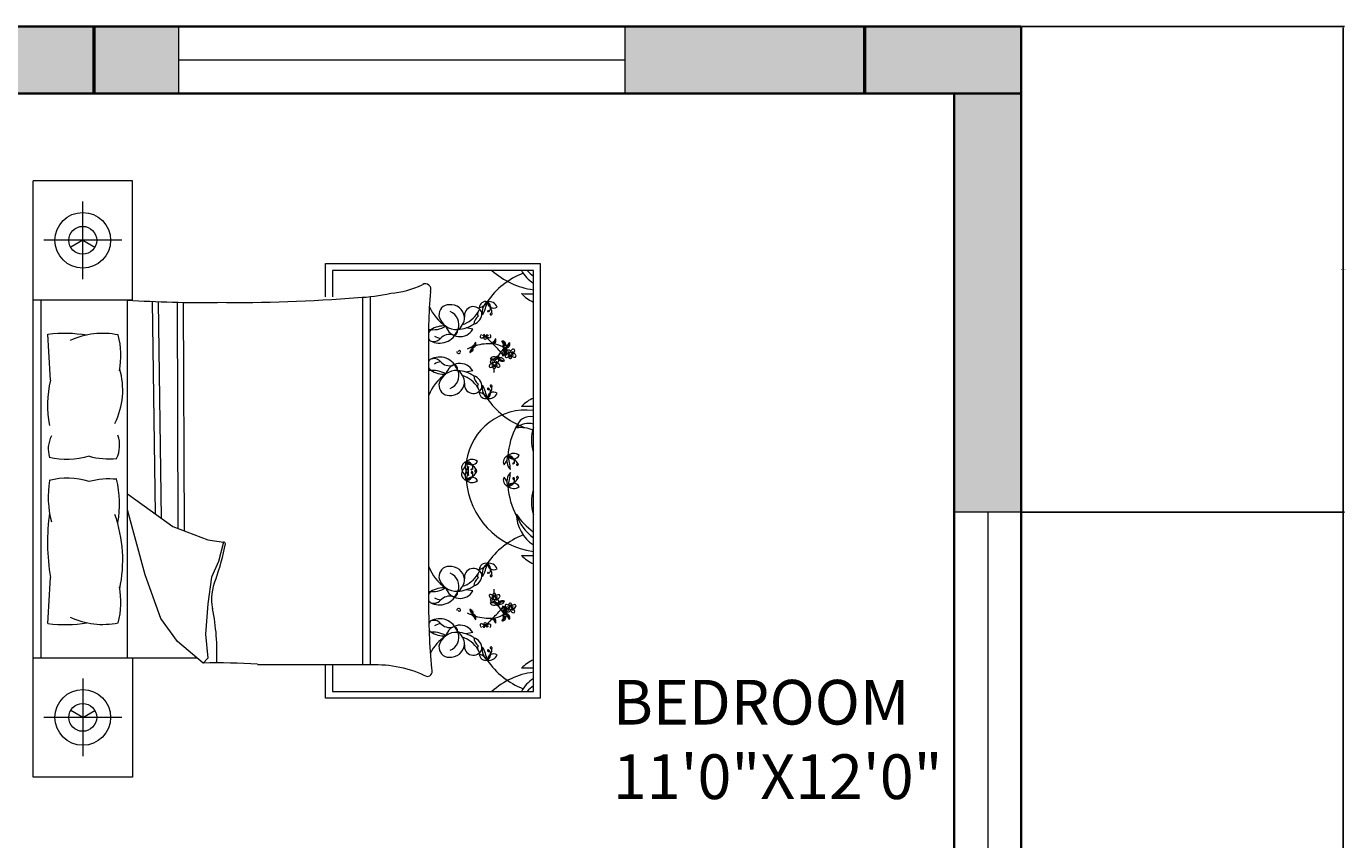
# Model space of a CAD drawing. Units: inches. Extents: x -28 to 485, y -861 to 54.
# Tile 14 of 14: x 308 to 485, y -99 to 10. Entities that reach past the tile are written whole.
import ezdxf

# ---------------------------------------------------------------- set-up
doc = ezdxf.new("R2010")
doc.units = ezdxf.units.IN
doc.header["$MEASUREMENT"] = 0
for name, color, linetype, lineweight in [('A-ANNO-DIMS', 2, 'Continuous', 18), ('A-AREA-IDEN', 7, 'Continuous', 18), ('A-COLS', 7, 'Continuous', 50), ('A-COLS-PATT', 8, 'Continuous', 13), ('A-FURN', 8, 'Continuous', 13), ('A-GLAZ', 4, 'Continuous', 18), ('A-WALL', 7, 'Continuous', 35), ('A-WALL-PATT', 34, 'Continuous', 13)]:
    doc.layers.add(name, color=color, linetype=linetype, lineweight=lineweight)
doc.styles.get("Standard").update_dxf_attribs({"font": 'arial.ttf'})
doc.dimstyles.get("Standard").update_dxf_attribs({"dimtxt": 0.18, "dimasz": 0.18, "dimexe": 0.18, "dimexo": 0.0625, "dimgap": 0.09, "dimtad": 0, "dimtih": 1, "dimtoh": 1, "dimdec": 0, "dimzin": 0, "dimdsep": 46, "dimlunit": 3, "dimtxsty": 'Standard', "dimcen": 0.09, "dimadec": 0, "dimazin": 0, "dimtfac": 1, "dimtdec": 0, "dimtofl": 0, "dimtmove": 0, "dimatfit": 3, "dimfxl": 1, "dimtolj": 1, "dimtzin": 0, "dimarcsym": 0})

# ---------------------------------------------------------------- blocks, each defined once
blk = doc.blocks.new('BED-DOUBLE-WITH-NIGHTSTANDS')
for p, q in [((0, 0), (0, 80.08)), ((6.67, 66.84), (6.67, 77.31)), ((11.91, 72.08), (1.44, 72.08)), ((39.26, 64.51), (39.26, 68.96)), ((39.26, 68.96), (68.11, 68.96)), ((40.19, 68.03), (40.19, 64.5)), ((67.18, 68.03), (40.19, 68.03)), ((67.18, 11.5), (67.18, 68.03)), ((68.11, 68.96), (68.11, 10.57)), ((1.03, 64.07), (1.03, 16.02)), ((12.66, 16.02), (12.66, 64.07)), ((15.98, 63.85), (16.38, 35.34)), ((16.8, 63.82), (17.22, 34.74)), ((19.33, 63.78), (19.45, 33.37)), ((20.15, 63.78), (20.27, 33.06)), ((44.25, 64.43), (44.25, 15.09)), ((45.25, 64.51), (45.25, 15.09)), ((59.06, 60.14), (58.15, 60.31)), ((53.12, 56.3), (53.12, 23.78)), ((59.06, 54.54), (58.15, 54.36)), ((12.66, 38.02), (18.76, 33.63)), ((15.04, 27.14), (12.66, 35.87)), ((18.76, 33.63), (23.47, 31.84)), ((23.47, 31.84), (25.57, 31.52)), ((25.57, 31.52), (24.92, 28.93)), ((24.92, 28.93), (23.95, 26.82)), ((17.14, 21.3), (15.04, 27.14)), ((23.95, 26.82), (23.47, 23.25)), ((59.06, 24.99), (58.15, 25.16)), ((23.47, 23.25), (23.14, 19.19)), ((19.41, 18.22), (17.14, 21.3)), ((22.82, 15.3), (19.41, 18.22)), ((23.14, 19.19), (23.47, 15.95)), ((59.06, 19.39), (58.15, 19.21)), ((0, 16.02), (21.98, 16.02)), ((23.47, 15.95), (22.82, 15.3)), ((39.26, 10.57), (39.26, 15.1)), ((40.19, 15.1), (40.19, 11.5)), ((6.67, 13.24), (6.67, 2.78)), ((40.19, 11.5), (67.18, 11.5)), ((68.11, 10.57), (39.26, 10.57)), ((11.91, 8.01), (1.44, 8.01))]:
    blk.add_line(p, q)
for points in [[(0, 64.07), (13.35, 64.07), (13.35, 80.08), (0, 80.08)], [(6.67, 72.08), (5.06, 71.14)], [(6.67, 72.08), (8.29, 71.14)], [(13.35, 16.02), (13.35, 0), (0, 0)], [(6.67, 8.01), (5.06, 8.94)], [(6.67, 8.01), (8.29, 8.94)]]:
    blk.add_lwpolyline(points)
for points in [[(43.62, 64.41, 0.056112), (48.03, 64.99, 0.095341), (52.27, 66.12)], [(2, 59.47, -0.074897), (7.23, 59.37, 0.472817)], [(7.52, 43.09, -0.14099), (2.18, 42.93, -0.235245)], [(7.52, 39.67, 0.14099), (2.18, 39.83, 0.235245)], [(2, 20.62, 0.074897), (7.23, 20.71, -0.472817)], [(30.15, 15.13, 0.001242), (45.35, 15.09, -0.127202), (52.92, 13.49)]]:
    blk.add_lwpolyline(points, format="xyb")
for centre, radius in [((6.67, 72.08), 3.74), ((6.67, 72.08), 1.87), ((64.11, 56.84), 0.204), ((61.96, 55.51), 0.204), ((61.96, 24.02), 0.204), ((64.11, 22.68), 0.204), ((6.67, 8.01), 3.74), ((6.67, 8.01), 1.87)]:
    blk.add_circle(centre, radius)
for centre, radius, start, end in [((69.62, 57.92), 10.46, 111.4092, 145.6135), ((68.59, 75.81), 10.46, 228.1144, 262.255), ((69.99, 70.57), 5.1, 209.8884, 236.5383), ((70.94, 72.4), 6.35, 223.5186, 233.6964), ((52.68, 65.51), 0.73, 336.5219, 123.8264), ((22.44, 207.63), 143.9, 266.1, 270.9282), ((27.68, 251.44), 187.71, 269.1145, 274.8735), ((131.01, 58.75), 77.93, 175.2402, 181.8035), ((60.79, 62.99), 0.867, 76.272, 177.0484), ((59.47, 64.76), 1.79, 284.7031, 328.6173), ((61.96, 62.49), 1.65, 125.7657, 194.5347), ((53.85, 65.41), 7.32, 332.8176, 347.4827), ((61.24, 62.69), 1.16, 20.9613, 102.2885), ((61.86, 63.85), 0.873, 181.7131, 301.5367), ((59, 62.09), 2.64, 2.0648, 41.1598), ((60.59, 63.07), 0.856, 316.2238, 62.3173), ((68.81, 67.71), 4.25, 221.0454, 247.4453), ((66.52, 79.36), 14.47, 266.3481, 272.5919), ((58.76, 65.61), 6.06, 203.6453, 236.3329), ((55.85, 62.08), 1.35, 88.9462, 185.5144), ((56.04, 61.53), 1.91, 7.1143, 95.0551), ((55.32, 60.77), 1.86, 338.5779, 68.4181), ((56.48, 64.35), 3.78, 288.2955, 328.7386), ((59.12, 61.97), 1.2, 19.1312, 189.736), ((58.76, 62.26), 1.5, 285.6955, 4.031), ((60.43, 62.21), 0.737, 126.7319, 206.0245), ((61.09, 62.57), 0.0682, 20.2667, 316.2271), ((61.51, 62.18), 0.13, 168.5166, 2.0648), ((61.45, 62.19), 0.0631, 52.0591, 168.5166), ((53.71, 63.39), 3.32, 259.249, 301.1782), ((55.15, 57.49), 3.09, 85.2696, 124.215), ((56.85, 62.5), 2.41, 193.079, 274.7067), ((57.33, 61.13), 1.99, 196.8663, 330.0915), ((55.62, 61.86), 2.33, 305.9599, 357.6409), ((56.78, 64.39), 4.3, 273.4924, 303.7117), ((60.76, 60.64), 1.6, 128.4175, 173.8338), ((-760.15, 15.33), 763.42, 2.85022, 3.31479), ((9.33, 49.26), 10.32, 78.2417, 114.8684), ((1.06, 56.61), 10.73, 348.9631, 14.8961), ((54, 59.28), 0.964, 127.675, 162.5814), ((54, 59.28), 0.964, 196.6343, 225.5483), ((54.57, 60.82), 2.55, 240.8249, 340.7178), ((53.81, 59.69), 1.2, 246.1646, 318.4347), ((55.03, 61.2), 2.3, 240.0851, 262.564), ((55.94, 57.8), 1.64, 74.8529, 138.4347), ((56.5, 59.87), 0.497, 254.8529, 12.6959), ((55.15, 57.49), 3.09, 53.6555, 57.2989), ((60.19, 59.12), 0.158, 125.0752, 284.7644), ((60.43, 59.18), 0.34, 127.3642, 168.4363), ((60.17, 59.45), 0.49, 277.4968, 341.2737), ((60.56, 59.22), 0.195, 88.1325, 178.8919), ((60.95, 59.02), 0.422, 136.3462, 189.6513), ((60.71, 58.98), 0.176, 189.6513, 312.3208), ((60.75, 59.46), 0.204, 183.2768, 356.7232), ((61.39, 59.1), 0.668, 164.2829, 186.9148), ((60.6, 59.09), 0.334, 312.3208, 40.2111), ((61.31, 59.47), 0.474, 201.6382, 274.947), ((60.68, 58.82), 0.619, 42.3896, 66.5724), ((66.93, 63.72), 7.6, 217.9541, 226.8459), ((61.13, 59.18), 0.337, 10.9597, 52.2379), ((61.33, 59.15), 0.156, 274.947, 37.5263), ((61.75, 58.56), 0.384, 265.7131, 351.6568), ((60.91, 59.35), 1.29, 313.6929, 321.7899), ((62.33, 58.47), 0.42, 115.5379, 168.6744), ((60.9, 59.07), 1.27, 329.344, 349.7412), ((59.89, 58.78), 2.26, 352.8698, 1.6736), ((63.07, 58.33), 0.228, 33.0979, 123.1364), ((58.05, 55.12), 5.96, 31.1156, 34.8118), ((62.74, 57.94), 0.617, 2.3172, 70.5201), ((57.16, 57.12), 0.251, 169.5864, 349.5616), ((57.25, 57.11), 0.154, 349.5616, 167.2949), ((61.28, 51.56), 6.63, 110.1059, 116.9968), ((59.06, 57.02), 0.42, 129.5056, 182.6421), ((57.85, 58), 1.27, 308.4388, 328.836), ((57.63, 59.02), 2.26, 296.5064, 305.3102), ((57.61, 57.86), 1.29, 336.3901, 344.4871), ((59.01, 57.53), 0.163, 83.9457, 185.6216), ((58.36, 57.69), 0.671, 328.836, 0.8141), ((58.71, 57.49), 0.384, 306.5232, 32.4668), ((59.16, 57.79), 0.163, 112.5583, 214.2343), ((59.06, 58.08), 0.384, 265.7131, 351.6568), ((58.72, 58.29), 0.671, 297.3659, 329.344), ((58.21, 58.87), 1.29, 313.6929, 321.7899), ((59.64, 57.99), 0.42, 115.5379, 168.6744), ((58.21, 58.6), 1.27, 329.344, 349.7412), ((61.28, 51.56), 6.63, 86.1723, 106.4158), ((57.2, 58.31), 2.26, 352.8698, 1.6736), ((61.86, 58.27), 0.163, 112.5583, 214.2343), ((61.42, 58.77), 0.671, 297.3659, 329.344), ((61.45, 54.86), 3.33, 60.7959, 85.244), ((54.37, 50.07), 10.94, 37.8256, 47.7588), ((65.87, 54.52), 3.99, 130.182, 149.456), ((63.67, 56.79), 0.658, 139.3812, 199.9959), ((62.44, 57.27), 0.93, 310.9365, 22.7695), ((62.87, 57.22), 0.675, 285.6484, 332.2957), ((63.25, 57.78), 0.178, 135.7354, 318.1297), ((62.95, 58.07), 0.236, 315.7354, 31.1156), ((62.75, 57.57), 0.547, 319.3812, 5.5456), ((63.38, 57.79), 0.178, 68.2452, 250.6395), ((62.97, 58), 0.531, 352.6008, 57.1845), ((64.87, 54.44), 3.55, 111.7087, 116.2181), ((61.45, 54.86), 3.33, 47.5083, 55.9967), ((63.48, 58.12), 0.531, 252.8042, 349.6943), ((62.97, 57.17), 0.565, 331.1838, 51.6792), ((63.53, 58.17), 0.236, 248.2452, 323.6254), ((63.8, 56.56), 0.34, 93.635, 168.4363), ((63.33, 58.31), 0.617, 291.7087, 3.0299), ((63.75, 57.1), 0.2, 138.2946, 276.2474), ((63.83, 57.07), 0.278, 358.5719, 143.8954), ((58.93, 61.56), 5.96, 323.6254, 327.3216), ((63.92, 56.61), 0.195, 88.1325, 178.8919), ((63.99, 57.29), 0.281, 208.8493, 269.9355), ((63.75, 57.22), 0.321, 274.2123, 318.1587), ((63.81, 58.16), 0.228, 325.6077, 55.6462), ((64.73, 56.9), 0.643, 121.9501, 165.2442), ((64.28, 57.14), 0.135, 262.868, 7.094), ((64.04, 56.2), 0.619, 42.3896, 66.5724), ((64.27, 57.26), 0.403, 278.5614, 22.5914), ((64.49, 56.56), 0.337, 10.9597, 118.7804), ((64.49, 57.27), 0.202, 44.3732, 121.9501), ((54, 55.39), 0.964, 134.4517, 156.7144), ((54, 55.39), 0.964, 203.2856, 232.325), ((54.57, 53.85), 2.55, 19.2822, 119.1751), ((53.81, 54.99), 1.2, 41.5653, 113.8354), ((55.03, 53.47), 2.3, 97.436, 119.9149), ((55.94, 56.87), 1.64, 221.5653, 285.1471), ((57.33, 53.55), 1.99, 29.9085, 163.1337), ((56.5, 54.81), 0.497, 347.3041, 105.1471), ((61.4, 55.17), 0.158, 125.0752, 284.7644), ((61.65, 55.23), 0.34, 93.635, 168.4363), ((61.66, 57.07), 0.93, 253.6301, 325.4631), ((61.92, 55.78), 0.658, 82.0748, 142.6895), ((61.85, 56.68), 0.675, 228.342, 274.9894), ((61.6, 55.76), 0.2, 138.2946, 276.2474), ((61.38, 55.5), 0.49, 277.4968, 341.2737), ((61.68, 55.73), 0.278, 358.5719, 143.8954), ((61.77, 55.27), 0.195, 88.1325, 178.8919), ((61.84, 55.95), 0.281, 208.8493, 269.9355), ((61.6, 55.89), 0.321, 274.2123, 318.1587), ((62.16, 55.06), 0.422, 136.3462, 189.6513), ((61.92, 55.02), 0.176, 189.6513, 312.3208), ((61.87, 56.57), 0.565, 273.8774, 357.1501), ((62.6, 55.14), 0.668, 164.2829, 186.9148), ((62.58, 55.56), 0.643, 121.9501, 165.2442), ((62.09, 56.97), 0.547, 262.0748, 308.2393), ((61.81, 55.14), 0.334, 312.3208, 40.2111), ((62.52, 55.52), 0.474, 201.6382, 274.947), ((62.13, 55.81), 0.135, 262.868, 7.094), ((61.89, 54.87), 0.619, 42.3896, 66.5724), ((62.12, 55.92), 0.403, 278.5614, 22.5914), ((62.34, 55.23), 0.337, 10.9597, 118.7804), ((65.87, 54.52), 3.99, 156.1523, 156.9499), ((62.34, 55.94), 0.202, 44.3732, 121.9501), ((62.97, 56.41), 0.565, 181.4625, 249.4747), ((62.87, 56.86), 0.547, 215.1128, 261.2773), ((63.31, 56.83), 0.93, 197.889, 269.722), ((62.55, 55.2), 0.156, 274.947, 37.5263), ((63.02, 56.51), 0.675, 248.3627, 295.0101), ((62.69, 55.67), 0.658, 20.6625, 81.2773), ((63.55, 56.5), 0.158, 125.0752, 284.7644), ((63.53, 56.83), 0.49, 277.4968, 341.2737), ((64.31, 56.4), 0.422, 136.3462, 189.6513), ((64.07, 56.36), 0.176, 189.6513, 312.3208), ((64.75, 56.48), 0.668, 164.2829, 186.9148), ((63.96, 56.47), 0.334, 312.3208, 40.2111), ((64.67, 56.85), 0.474, 201.6382, 274.947), ((64.7, 56.53), 0.156, 274.947, 37.5263), ((16.01, 49.96), 14.08, 166.3427, 191.1841), ((1.85, 51.98), 10.19, 333.8761, 16.1746), ((53.71, 51.28), 3.32, 58.8218, 100.2867), ((58.76, 49.06), 6.06, 123.6671, 158.5059), ((55.15, 57.18), 3.09, 235.785, 274.7304), ((56.85, 52.18), 2.41, 85.2933, 166.921), ((55.32, 53.9), 1.86, 291.5819, 21.4221), ((55.15, 57.18), 3.09, 302.7011, 306.3445), ((55.62, 52.81), 2.33, 2.3591, 54.0401), ((56.78, 50.29), 4.3, 56.2883, 86.5076), ((56.48, 50.32), 3.78, 31.2614, 71.7045), ((60.76, 54.03), 1.6, 186.1662, 231.5825), ((58.76, 52.42), 1.5, 355.969, 74.3045), ((65.87, 54.52), 3.99, 175.2415, 182.8929), ((55.85, 52.59), 1.35, 174.4856, 271.0538), ((56.04, 53.15), 1.91, 264.9449, 352.8857), ((59.12, 52.71), 1.2, 170.264, 340.8688), ((60.43, 52.46), 0.737, 153.9755, 233.2681), ((60.79, 51.69), 0.867, 182.9516, 283.728), ((59.47, 49.92), 1.79, 31.3827, 75.2969), ((61.96, 52.19), 1.65, 165.4653, 234.2343), ((53.85, 49.26), 7.32, 12.5173, 27.1824), ((59, 52.59), 2.64, 318.8402, 357.9352), ((60.59, 51.6), 0.856, 297.6827, 43.7762), ((61.86, 50.82), 0.873, 58.4633, 178.2869), ((61.24, 51.98), 1.16, 257.7115, 339.0387), ((61.13, 52.12), 0.113, 43.7762, 339.7183), ((61.51, 52.5), 0.13, 357.9352, 191.4834), ((61.45, 52.48), 0.0631, 191.4834, 307.9409), ((69.62, 56.75), 10.46, 214.3865, 248.5908), ((68.81, 46.96), 4.25, 112.5547, 138.9546), ((66.52, 35.31), 14.47, 87.4081, 93.6519), ((66.17, 41.19), 8.09, 82.8636, 171.8197), ((66.74, 46.53), 1.88, 76.3898, 169.0739), ((74.19, 42.33), 10.46, 152.5854, 175.5377), ((66.48, 45.12), 2.37, 72.8609, 131.9049), ((65.43, 42.24), 4.68, 68.117, 96.6195), ((72.68, 45.26), 5.75, 162.9798, 196.4569), ((5.99, 44.03), 3.96, 153.3437, 196.1026), ((7.37, 44.56), 4.25, 335.0183, 18.5407), ((10.2, 52.53), 9.81, 254.1707, 275.9871), ((58.94, 41.49), 1.16, 50.8855, 132.2127), ((64.01, 42.31), 0.867, 106.1963, 206.9726), ((61.98, 43.19), 1.79, 314.6273, 358.5415), ((65.27, 42.46), 1.65, 155.6899, 224.4589), ((64.54, 42.29), 1.16, 50.8855, 132.2127), ((64.51, 43.6), 0.873, 211.6373, 331.4609), ((63.8, 42.29), 0.856, 346.148, 92.2415), ((62.91, 40.64), 2.64, 31.989, 71.0841), ((56.78, 40.96), 7.32, 2.7418, 17.407), ((75.64, 42.98), 8.5, 174.3643, 175.6213), ((81.47, 38.5), 15.2, 160.0972, 160.2783), ((58.4, 41.51), 0.867, 106.1963, 206.9726), ((58.4, 40.68), 0.867, 153.0274, 253.8037), ((56.38, 42.39), 1.79, 314.6273, 358.5415), ((56.38, 39.81), 1.79, 1.4585, 45.3727), ((59.67, 41.66), 1.65, 155.6899, 224.4589), ((59.67, 40.53), 1.65, 135.5411, 204.3101), ((58.91, 42.8), 0.873, 211.6373, 331.4609), ((58.2, 41.49), 0.856, 346.148, 92.2415), ((57.3, 39.84), 2.64, 31.989, 71.0841), ((51.18, 40.16), 7.32, 2.7418, 17.407), ((51.18, 42.04), 7.32, 342.593, 357.2582), ((57.3, 42.35), 2.64, 288.9159, 328.011), ((58.2, 40.71), 0.856, 267.7585, 13.852), ((58.87, 41.3), 0.0682, 50.1909, 346.0209), ((58.92, 40.88), 0.113, 13.852, 309.9245), ((59.44, 41.17), 0.13, 198.4408, 31.989), ((59.37, 41.15), 0.0631, 81.9833, 198.4408), ((59.44, 41.02), 0.13, 328.011, 161.5592), ((59.37, 41.04), 0.0631, 161.5592, 278.0167), ((65.27, 39.73), 1.65, 135.5411, 204.3101), ((56.78, 41.24), 7.32, 342.593, 357.2582), ((64.47, 42.1), 0.0682, 50.1909, 346.0209), ((64.98, 41.95), 0.0631, 81.9833, 198.4408), ((65.04, 41.98), 0.13, 198.4408, 31.989), ((16.3, 37.72), 14.27, 171.5249, 193.96), ((10.2, 30.23), 9.81, 84.0129, 105.8293), ((-2.51, 36.66), 14.12, 349.8617, 13.6238), ((58.91, 39.39), 0.873, 28.5391, 148.3627), ((58.94, 40.71), 1.16, 227.7873, 309.1145), ((68.59, 40.66), 10.46, 184.4623, 262.255), ((64.01, 39.88), 0.867, 153.0274, 253.8037), ((61.98, 39.01), 1.79, 1.4585, 45.3727), ((62.91, 41.55), 2.64, 288.9159, 328.011), ((63.8, 39.91), 0.856, 267.7585, 13.852), ((64.51, 38.59), 0.873, 28.5391, 148.3627), ((64.54, 39.91), 1.16, 227.7873, 309.1145), ((74.19, 39.86), 10.46, 184.4623, 207.4146), ((64.52, 40.08), 0.113, 13.852, 309.9245), ((64.98, 40.24), 0.0631, 161.5592, 278.0167), ((65.04, 40.22), 0.13, 328.011, 161.5592), ((72.68, 36.94), 5.75, 163.5431, 197.0202), ((75.64, 39.22), 8.5, 184.3787, 185.6357), ((81.47, 43.7), 15.2, 199.7217, 199.9028), ((30.98, 31.59), 29.04, 172.2196, 189.497), ((-6.57, 29.12), 18.61, 348.0397, 19.2615), ((69.99, 35.42), 5.1, 181.272, 236.5383), ((72.72, 40.59), 9.45, 214.0123, 234.053), ((70.94, 37.25), 6.35, 197.8504, 233.6964), ((69.62, 22.77), 10.46, 111.4092, 145.6135), ((-4.69, 37.08), 31.06, 340.1194, 349.3383), ((25.64, 31.34), 0.193, 358.8623, 109.7536), ((60.79, 27.84), 0.867, 76.272, 177.0484), ((59.47, 29.61), 1.79, 284.7031, 328.6173), ((61.96, 27.34), 1.65, 125.7657, 194.5347), ((53.85, 30.27), 7.32, 332.8176, 347.4827), ((61.24, 27.55), 1.16, 20.9613, 102.2885), ((60.59, 27.92), 0.856, 316.2238, 62.3173), ((59, 26.94), 2.64, 2.0648, 41.1598), ((61.86, 28.71), 0.873, 181.7131, 301.5367), ((66.52, 44.21), 14.47, 266.3481, 272.5919), ((68.81, 32.56), 4.25, 221.0454, 247.4453), ((-760.15, 64.76), 763.42, 356.68521, 357.14978), ((58.76, 30.46), 6.06, 201.4941, 236.3329), ((55.85, 26.93), 1.35, 88.9462, 185.5144), ((56.85, 27.35), 2.41, 193.079, 274.7067), ((56.04, 26.38), 1.91, 7.1143, 95.0551), ((55.32, 25.63), 1.86, 338.5779, 68.4181), ((55.62, 26.71), 2.33, 305.9599, 357.6409), ((56.48, 29.2), 3.78, 288.2955, 328.7386), ((59.12, 26.82), 1.2, 19.1312, 189.736), ((58.76, 27.11), 1.5, 285.6955, 4.031), ((60.76, 25.49), 1.6, 128.4175, 173.8338), ((60.43, 27.07), 0.737, 126.7319, 206.0245), ((61.09, 27.42), 0.0682, 20.2667, 316.2271), ((61.51, 27.03), 0.13, 168.5166, 2.0648), ((61.45, 27.04), 0.0631, 52.0591, 168.5166), ((1.06, 23.47), 10.73, 345.1039, 11.0369), ((30.48, 23.89), 6.52, 156.2616, 191.3392), ((53.71, 28.24), 3.32, 259.7133, 301.1782), ((54, 24.13), 0.964, 127.675, 156.7144), ((54.57, 25.67), 2.55, 240.8249, 340.7178), ((55.15, 22.34), 3.09, 85.2696, 124.215), ((57.33, 25.98), 1.99, 196.8663, 330.0915), ((56.5, 24.72), 0.497, 254.8529, 12.6959), ((55.15, 22.34), 3.09, 53.6555, 57.2989), ((56.78, 29.24), 4.3, 273.4924, 303.7117), ((65.87, 25.01), 3.99, 177.1071, 184.7585), ((136.48, 22.83), 83.37, 179.3433, 185.6887), ((54, 24.13), 0.964, 203.229, 225.5483), ((53.81, 24.54), 1.2, 246.1646, 318.4347), ((55.03, 26.06), 2.3, 240.0851, 262.564), ((55.94, 22.65), 1.64, 74.8529, 138.4347), ((61.4, 24.36), 0.158, 75.2356, 234.9248), ((61.65, 24.3), 0.34, 191.5637, 266.365), ((61.6, 23.76), 0.2, 83.7526, 221.7054), ((61.85, 22.84), 0.675, 85.0106, 131.658), ((61.66, 22.46), 0.93, 34.5369, 106.3699), ((61.92, 23.75), 0.658, 217.3105, 277.9252), ((61.38, 24.03), 0.49, 18.7263, 82.5032), ((61.68, 23.79), 0.278, 216.1046, 1.4281), ((61.77, 24.25), 0.195, 181.1081, 271.8675), ((61.84, 23.57), 0.281, 90.0645, 151.1507), ((61.6, 23.64), 0.321, 41.8413, 85.7877), ((61.92, 24.5), 0.176, 47.6792, 170.3487), ((62.16, 24.46), 0.422, 170.3487, 223.6538), ((61.87, 22.95), 0.565, 2.8499, 86.1226), ((62.6, 24.38), 0.668, 173.0852, 195.7171), ((62.58, 23.96), 0.643, 194.7558, 238.0499), ((62.09, 22.55), 0.547, 51.7607, 97.9252), ((61.81, 24.39), 0.334, 319.7889, 47.6792), ((62.52, 24.01), 0.474, 85.053, 158.3618), ((62.13, 23.71), 0.135, 352.906, 97.132), ((61.89, 24.66), 0.619, 293.4276, 317.6104), ((62.34, 24.29), 0.337, 241.2196, 349.0403), ((62.12, 23.6), 0.403, 337.4086, 81.4386), ((65.87, 25.01), 3.99, 203.0501, 203.8477), ((62.34, 23.59), 0.202, 238.0499, 315.6268), ((62.97, 23.11), 0.565, 110.5253, 178.5375), ((63.31, 22.7), 0.93, 90.278, 162.111), ((62.87, 22.67), 0.547, 98.7227, 144.8872), ((62.55, 24.33), 0.156, 322.4737, 85.053), ((63.02, 23.01), 0.675, 64.9899, 111.6373), ((62.69, 23.86), 0.658, 278.7227, 339.3375), ((63.55, 23.03), 0.158, 75.2356, 234.9248), ((63.53, 22.69), 0.49, 18.7263, 82.5032), ((64.07, 23.17), 0.176, 47.6792, 170.3487), ((64.31, 23.13), 0.422, 170.3487, 223.6538), ((64.75, 23.05), 0.668, 173.0852, 195.7171), ((63.96, 23.05), 0.334, 319.7889, 47.6792), ((64.67, 22.68), 0.474, 85.053, 158.3618), ((64.7, 22.99), 0.156, 322.4737, 85.053), ((9.33, 30.82), 10.32, 245.1316, 281.7583), ((-5.54, 16.67), 30.23, 357.4519, 11.3392), ((57.16, 22.4), 0.251, 10.4384, 190.4136), ((57.25, 22.42), 0.154, 192.7051, 10.4384), ((61.28, 27.97), 6.63, 243.0032, 249.8941), ((57.85, 21.53), 1.27, 31.164, 51.5612), ((59.06, 22.5), 0.42, 177.3579, 230.4944), ((57.63, 20.5), 2.26, 54.6898, 63.4936), ((57.61, 21.66), 1.29, 15.5129, 23.6099), ((59.01, 21.99), 0.163, 174.3784, 276.0543), ((58.71, 22.03), 0.384, 327.5332, 53.4768), ((58.36, 21.84), 0.671, 359.1859, 31.164), ((59.16, 21.74), 0.163, 145.7657, 247.4417), ((59.06, 21.45), 0.384, 8.3432, 94.2869), ((58.72, 21.23), 0.671, 30.656, 62.6341), ((58.21, 20.66), 1.29, 38.2101, 46.3071), ((59.64, 21.53), 0.42, 191.3256, 244.4621), ((58.21, 20.93), 1.27, 10.2588, 30.656), ((61.28, 27.97), 6.63, 253.5842, 273.8277), ((57.2, 21.22), 2.26, 358.3264, 7.1302), ((66.93, 15.8), 7.6, 133.1541, 142.0459), ((61.86, 21.26), 0.163, 145.7657, 247.4417), ((54.37, 29.45), 10.94, 312.2412, 322.1744), ((61.45, 24.67), 3.33, 274.756, 299.2041), ((61.75, 20.97), 0.384, 8.3432, 94.2869), ((61.42, 20.76), 0.671, 30.656, 62.6341), ((65.87, 25.01), 3.99, 210.544, 229.818), ((62.74, 21.59), 0.617, 289.4799, 357.6828), ((58.05, 24.41), 5.96, 325.1882, 328.8844), ((63.67, 22.74), 0.658, 160.0041, 220.6188), ((62.44, 22.26), 0.93, 337.2305, 49.0635), ((62.87, 22.31), 0.675, 27.7043, 74.3516), ((63.25, 21.74), 0.178, 41.8703, 224.2646), ((62.95, 21.45), 0.236, 328.8844, 44.2646), ((62.75, 21.95), 0.547, 354.4544, 40.6188), ((63.38, 21.74), 0.178, 109.3605, 291.7548), ((62.97, 21.52), 0.531, 302.8155, 7.3992), ((64.87, 25.09), 3.55, 243.7819, 248.2913), ((61.45, 24.67), 3.33, 304.0033, 312.4917), ((62.97, 22.35), 0.565, 308.3208, 28.8162), ((63.48, 21.4), 0.531, 10.3057, 107.1958), ((63.53, 21.36), 0.236, 36.3746, 111.7548), ((63.8, 22.96), 0.34, 191.5637, 266.365), ((63.75, 22.43), 0.2, 83.7526, 221.7054), ((63.33, 21.21), 0.617, 356.9701, 68.2913), ((63.83, 22.46), 0.278, 216.1046, 1.4281), ((63.92, 22.92), 0.195, 181.1081, 271.8675), ((58.93, 17.96), 5.96, 32.6784, 36.3746), ((63.99, 22.24), 0.281, 90.0645, 151.1507), ((63.75, 22.31), 0.321, 41.8413, 85.7877), ((63.81, 21.37), 0.228, 304.3538, 34.3923), ((64.73, 22.63), 0.643, 194.7558, 238.0499), ((64.28, 22.38), 0.135, 352.906, 97.132), ((64.04, 23.32), 0.619, 293.4276, 317.6104), ((64.49, 22.96), 0.337, 241.2196, 349.0403), ((64.27, 22.27), 0.403, 337.4086, 81.4386), ((64.49, 22.25), 0.202, 238.0499, 315.6268), ((54, 20.25), 0.964, 134.4517, 153.558), ((54, 20.25), 0.964, 210.0293, 232.325), ((54.57, 18.71), 2.55, 19.2822, 119.1751), ((53.81, 19.84), 1.2, 41.5653, 113.8354), ((55.03, 18.32), 2.3, 97.436, 119.9149), ((55.94, 21.72), 1.64, 221.5653, 285.1471), ((57.33, 18.4), 1.99, 29.9085, 163.1337), ((56.5, 19.66), 0.497, 347.3041, 105.1471), ((55.15, 22.04), 3.09, 302.7011, 306.3445), ((55.62, 17.67), 2.33, 2.3591, 54.0401), ((60.19, 20.41), 0.158, 75.2356, 234.9248), ((60.43, 20.35), 0.34, 191.5637, 232.6358), ((60.17, 20.07), 0.49, 18.7263, 82.5032), ((60.56, 20.3), 0.195, 181.1081, 271.8675), ((60.71, 20.55), 0.176, 47.6792, 170.3487), ((60.95, 20.51), 0.422, 170.3487, 223.6538), ((60.75, 20.06), 0.204, 3.2768, 176.7232), ((61.39, 20.43), 0.668, 173.0852, 195.7171), ((60.6, 20.43), 0.334, 319.7889, 47.6792), ((61.31, 20.06), 0.474, 85.053, 158.3618), ((60.68, 20.7), 0.619, 293.4276, 317.6104), ((61.13, 20.34), 0.337, 307.7621, 349.0403), ((61.33, 20.37), 0.156, 322.4737, 85.053), ((60.91, 20.18), 1.29, 38.2101, 46.3071), ((62.33, 21.06), 0.42, 191.3256, 244.4621), ((60.9, 20.45), 1.27, 10.2588, 30.656), ((59.89, 20.74), 2.26, 358.3264, 7.1302), ((63.07, 21.2), 0.228, 236.8636, 326.9021), ((53.71, 16.14), 3.32, 58.8218, 99.1554), ((58.76, 13.91), 6.06, 123.6671, 153.2997), ((55.15, 22.04), 3.09, 235.785, 274.7304), ((56.85, 17.03), 2.41, 85.2933, 166.921), ((56.04, 18), 1.91, 264.9449, 352.8857), ((55.32, 18.75), 1.86, 291.5819, 21.4221), ((56.78, 15.14), 4.3, 56.2883, 86.5076), ((56.48, 15.18), 3.78, 31.2614, 71.7045), ((59.12, 17.56), 1.2, 170.264, 340.8688), ((58.76, 17.27), 1.5, 355.969, 74.3045), ((60.76, 18.89), 1.6, 186.1662, 231.5825), ((55.85, 17.44), 1.35, 174.4856, 271.0538), ((60.43, 17.31), 0.737, 153.9755, 233.2681), ((59.47, 14.77), 1.79, 31.3827, 75.2969), ((60.79, 16.54), 0.867, 182.9516, 283.728), ((61.96, 17.04), 1.65, 165.4653, 234.2343), ((53.85, 14.11), 7.32, 12.5173, 27.1824), ((59, 17.44), 2.64, 318.8402, 357.9352), ((60.59, 16.46), 0.856, 297.6827, 43.7762), ((61.86, 15.67), 0.873, 58.4633, 178.2869), ((61.24, 16.83), 1.16, 257.7115, 339.0387), ((61.13, 16.97), 0.113, 43.7762, 339.7183), ((61.51, 17.35), 0.13, 357.9352, 191.4834), ((61.45, 17.33), 0.0631, 191.4834, 307.9409), ((24.81, -58.13), 73.46, 85.8294, 91.553), ((52.87, 14.23), 0.739, 273.98, 27.3412), ((69.62, 21.6), 10.46, 214.3865, 248.5908), ((68.81, 11.81), 4.25, 112.5547, 138.9546), ((66.52, 0.17), 14.47, 87.4081, 93.6519), ((68.59, 3.71), 10.46, 97.745, 131.8856), ((69.99, 8.96), 5.1, 123.4617, 150.1116), ((70.94, 7.13), 6.35, 126.3036, 136.4814)]:
    blk.add_arc(centre, radius, start, end)
blk = doc.blocks.new('WINDOW-60IN')
for p, q in [((0, 60), (0, 0)), ((9, 60), (0, 60)), ((4.5, 60), (4.5, 0)), ((9, 0), (9, 60)), ((0, 0), (9, 0))]:
    blk.add_line(p, q)
blk = doc.blocks.new('*D53')
at = {"layer": 'A-ANNO-DIMS', "color": 0, "lineweight": -2, "transparency": 16777216}
for p, q in [((441.35, 10.13), (484.71, 10.13)), ((484.53, 9.95), (484.53, -403.68)), ((484.53, -817.69), (484.53, -404.05)), ((441.35, -817.87), (484.71, -817.87))]:
    blk.add_line(p, q, dxfattribs=at)
at = {"layer": 'A-ANNO-DIMS', "color": 0, "transparency": 16777216}
for points in [[(484.5, 9.95), (484.56, 9.95), (484.53, 10.13)], [(484.5, -817.69), (484.56, -817.69), (484.53, -817.87)]]:
    blk.add_solid(points, dxfattribs=at)
at = {"layer": 'Defpoints', "color": 0, "transparency": 16777216}
for p in [(441.28, 10.13), (441.28, -817.87), (484.53, -817.87)]:
    blk.add_point(p, dxfattribs=at)
at = {"layer": 'A-ANNO-DIMS', "color": 0, "transparency": 16777216, "insert": (484.53, -403.87), "char_height": 0.18, "attachment_point": 5}
blk.add_mtext('\\A1;828', dxfattribs=at)
blk = doc.blocks.new('*D58')
at = {"layer": 'A-ANNO-DIMS', "color": 0, "lineweight": -2, "transparency": 16777216}
for p, q in [((441.35, 10.13), (484.71, 10.13)), ((484.53, 9.95), (484.53, -22.3)), ((484.53, -54.92), (484.53, -22.66)), ((441.35, -55.1), (484.71, -55.1))]:
    blk.add_line(p, q, dxfattribs=at)
at = {"layer": 'A-ANNO-DIMS', "color": 0, "transparency": 16777216}
for points in [[(484.5, 9.95), (484.56, 9.95), (484.53, 10.13)], [(484.5, -54.92), (484.56, -54.92), (484.53, -55.1)]]:
    blk.add_solid(points, dxfattribs=at)
at = {"layer": 'Defpoints', "color": 0, "transparency": 16777216}
for p in [(441.28, 10.13), (441.28, -55.1), (484.53, -55.1)]:
    blk.add_point(p, dxfattribs=at)
at = {"layer": 'A-ANNO-DIMS', "color": 0, "transparency": 16777216, "insert": (484.53, -22.48), "char_height": 0.18, "attachment_point": 5}
blk.add_mtext('\\A1;65.23', dxfattribs=at)

msp = doc.modelspace()

# ---------------------------------------------------------------- hatches: boundary and pattern name
at = {"layer": 'A-COLS-PATT'}
h = msp.add_hatch(color=256, dxfattribs=at)
h.dxf.hatch_style = 1
h.paths.add_polyline_path([(36.285, 10.133), (15.285, 10.133), (15.285, 1.133), (36.285, 1.133)])
h.paths.add_polyline_path([(160.785, 10.133), (139.785, 10.133), (139.785, 1.133), (160.785, 1.133)])
h.paths.add_polyline_path([(316.785, 10.133), (295.785, 10.133), (295.785, 1.133), (316.785, 1.133)])
h.paths.add_polyline_path([(441.285, 10.133), (420.285, 10.133), (420.285, 1.133), (441.285, 1.133)])
h.paths.add_polyline_path([(441.285, -138.367), (432.285, -138.367), (420.285, -138.367), (420.285, -147.367), (441.285, -147.367)])
h.paths.add_polyline_path([(304.785, -130.867), (295.785, -130.867), (295.785, -147.367), (304.785, -147.367), (304.785, -142.867)])
h.paths.add_polyline_path([(160.785, -130.867), (151.785, -130.867), (151.785, -142.867), (151.785, -147.367), (160.785, -147.367)])
h.paths.add_polyline_path([(36.285, -138.367), (24.285, -138.367), (15.285, -138.367), (15.285, -147.367), (36.285, -147.367)])
h.paths.add_polyline_path([(36.285, -355.867), (15.285, -355.867), (15.285, -364.867), (36.285, -364.867)])
h.paths.add_polyline_path([(160.785, -355.867), (139.785, -355.867), (139.785, -364.867), (160.785, -364.867)])
h.paths.add_polyline_path([(316.785, -355.867), (300.285, -355.867), (295.785, -355.867), (295.785, -364.867), (316.785, -364.867)])
at = {"layer": 'A-WALL-PATT'}
h = msp.add_hatch(color=256, dxfattribs=at)
h.dxf.hatch_style = 1
h.paths.add_polyline_path([(160.785, -808.867), (160.785, -817.867), (295.785, -817.867), (295.785, -808.867)])
h.paths.add_polyline_path([(316.785, -817.867), (323.776, -817.867), (323.776, -808.867), (316.785, -808.867)])
h.paths.add_polyline_path([(420.285, -817.867), (420.285, -808.867), (383.776, -808.867), (383.776, -817.867)])
h.paths.add_polyline_path([(432.285, -808.867), (441.285, -808.867), (441.285, -702.966), (432.285, -702.966), (432.285, -708.367), (397.785, -708.367), (397.785, -710.617), (397.785, -712.867), (432.285, -712.867)])
h.paths.add_polyline_path([(300.285, -712.867), (329.285, -712.867), (329.285, -710.617), (329.285, -708.367), (295.785, -708.367), (295.785, -808.867), (300.285, -808.867)])
h.paths.add_polyline_path([(160.785, -698.867), (158.535, -698.867), (156.285, -698.867), (156.285, -808.867), (160.785, -808.867)])
h.paths.add_polyline_path([(36.285, -808.867), (36.285, -817.867), (79.721, -817.867), (79.721, -808.867)])
h.paths.add_polyline_path([(15.285, -808.867), (24.285, -808.867), (24.285, -739.09), (15.285, -739.09)])
h.paths.add_polyline_path([(24.285, -640.781), (15.285, -640.781), (15.285, -679.09), (24.285, -679.09), (24.285, -664.867), (89.285, -664.867), (89.285, -662.617), (89.285, -660.367), (24.285, -660.367)])
h.paths.add_polyline_path([(15.285, -616.781), (24.285, -616.781), (24.285, -600.367), (15.285, -600.367)])
h.paths.add_polyline_path([(36.285, -595.867), (36.285, -600.367), (123.285, -600.367), (123.285, -660.367), (117.285, -660.367), (117.285, -664.867), (156.285, -664.867), (156.285, -670.867), (160.785, -670.867), (160.785, -660.367), (127.785, -660.367), (127.785, -600.367), (129.785, -600.367), (129.785, -598.117), (129.785, -595.867)])
h.paths.add_polyline_path([(367.785, -664.867), (363.285, -664.867), (363.285, -708.367), (357.285, -708.367), (357.285, -712.867), (369.785, -712.867), (369.785, -708.367), (367.785, -708.367)])
h.paths.add_polyline_path([(432.285, -664.867), (432.285, -666.966), (441.285, -666.966), (441.285, -642.367), (432.285, -642.367), (432.285, -660.367), (328.785, -660.367), (328.785, -664.867), (363.285, -664.867)])
h.paths.add_polyline_path([(333.285, -600.367), (420.285, -600.367), (420.285, -595.867), (326.785, -595.867), (326.785, -600.367), (328.785, -600.367), (328.785, -630.367), (331.035, -630.367), (333.285, -630.367)])
h.paths.add_polyline_path([(441.285, -600.367), (432.285, -600.367), (432.285, -618.367), (441.285, -618.367)])
h.paths.add_polyline_path([(432.285, -591.367), (441.285, -591.367), (441.285, -547.793), (432.285, -547.793)])
h.paths.add_polyline_path([(295.785, -588.367), (300.238, -588.367), (300.285, -583.867), (300.285, -451.867), (295.785, -451.867)])
h.paths.add_polyline_path([(420.285, -451.867), (420.285, -442.867), (316.785, -442.867), (316.785, -451.867)])
h.paths.add_polyline_path([(432.285, -487.793), (441.285, -487.793), (441.285, -451.867), (432.285, -451.867)])
h.paths.add_polyline_path([(432.285, -442.867), (441.285, -442.867), (441.285, -364.867), (432.285, -364.867)])
h.paths.add_polyline_path([(261.785, -451.867), (261.785, -447.367), (261.785, -444.758), (261.785, -442.867), (160.785, -442.867), (160.785, -451.867)])
h.paths.add_polyline_path([(139.785, -451.867), (139.785, -442.867), (36.285, -442.867), (36.285, -451.867)])
h.paths.add_polyline_path([(15.285, -491.617), (24.285, -491.617), (24.285, -451.867), (15.285, -451.867)])
h.paths.add_polyline_path([(24.285, -551.617), (15.285, -551.617), (15.285, -591.367), (24.285, -591.367)])
h.paths.add_polyline_path([(160.785, -451.867), (156.285, -451.867), (156.285, -588.367), (160.785, -588.367)])
h.paths.add_polyline_path([(139.785, -364.867), (139.785, -355.867), (36.285, -355.867), (36.285, -364.867)])
h.paths.add_polyline_path([(24.285, -364.867), (15.285, -364.867), (15.285, -373.867), (24.285, -373.867)])
h.paths.add_polyline_path([(15.285, -433.867), (15.285, -442.867), (24.285, -442.867), (24.285, -433.867)])
h.paths.add_polyline_path([(261.785, -364.867), (261.785, -360.367), (261.785, -355.867), (160.785, -355.867), (160.785, -364.867)])
h.paths.add_polyline_path([(295.785, -355.867), (289.785, -355.867), (289.785, -364.867), (295.785, -364.867)])
h.paths.add_polyline_path([(295.785, -355.867), (300.285, -355.867), (300.285, -259.867), (333.285, -259.867), (333.285, -257.617), (333.285, -255.367), (300.285, -255.367), (300.285, -207.367), (295.785, -207.367)])
h.paths.add_polyline_path([(420.285, -364.867), (420.285, -355.867), (316.785, -355.867), (316.785, -364.867)])
h.paths.add_polyline_path([(24.285, -311.192), (15.285, -311.192), (15.285, -355.867), (24.285, -355.867)])
h.paths.add_polyline_path([(24.285, -211.867), (54.144, -211.867), (54.144, -207.367), (24.285, -207.367), (24.285, -187.772), (15.285, -187.772), (15.285, -251.192), (24.285, -251.192)])
h.paths.add_polyline_path([(82.144, -207.367), (82.144, -209.617), (82.144, -211.867), (127.785, -211.867), (127.785, -147.367), (129.785, -147.367), (129.785, -145.117), (129.785, -142.867), (36.285, -142.867), (36.285, -147.367), (123.285, -147.367), (123.285, -207.367)])
h.paths.add_polyline_path([(160.785, -207.367), (156.285, -207.367), (156.285, -355.867), (160.785, -355.867)])
h.paths.add_polyline_path([(24.285, 1.133), (15.285, 1.133), (15.285, -54.408), (24.285, -54.408)])
h.paths.add_polyline_path([(36.285, 10.133), (36.285, 1.133), (70.235, 1.133), (70.235, 10.133)])
h.paths.add_polyline_path([(15.285, -138.367), (24.285, -138.367), (24.285, -114.408), (15.285, -114.408)])
h.paths.add_polyline_path([(24.285, -147.367), (15.285, -147.367), (15.285, -163.772), (24.285, -163.772)])
h.paths.add_polyline_path([(156.285, -130.867), (160.785, -130.867), (160.785, 1.133), (156.285, 1.133)])
h.paths.add_polyline_path([(130.235, 1.133), (139.785, 1.133), (139.785, 10.133), (130.235, 10.133)])
h.paths.add_polyline_path([(316.785, 10.133), (316.785, 1.133), (328.097, 1.133), (328.097, 10.133)])
h.paths.add_polyline_path([(300.285, 1.133), (295.785, 1.133), (295.785, -130.867), (300.285, -130.867)])
h.paths.add_polyline_path([(420.285, -147.367), (420.285, -142.867), (326.785, -142.867), (326.785, -145.117), (326.785, -147.367), (328.785, -147.367), (328.785, -177.367), (331.035, -177.367), (333.285, -177.367), (333.285, -147.367)])
h.paths.add_polyline_path([(333.285, -207.367), (333.285, -205.367), (328.785, -205.367), (328.785, -211.867), (363.285, -211.867), (363.285, -255.367), (361.285, -255.367), (361.285, -259.867), (369.785, -259.867), (369.785, -255.367), (367.785, -255.367), (367.785, -211.867), (432.285, -211.867), (432.285, -214.893), (441.285, -214.893), (441.285, -188.008), (432.285, -188.008), (432.285, -207.367)])
h.paths.add_polyline_path([(441.285, -250.893), (432.285, -250.893), (432.285, -255.367), (397.785, -255.367), (397.785, -257.617), (397.785, -259.867), (432.285, -259.867), (432.285, -355.867), (441.285, -355.867)])
h.paths.add_polyline_path([(432.285, -138.367), (441.285, -138.367), (441.285, -115.099), (432.285, -115.099)])
h.paths.add_polyline_path([(441.285, -147.367), (432.285, -147.367), (432.285, -164.008), (441.285, -164.008)])
h.paths.add_polyline_path([(420.285, 1.133), (420.285, 10.133), (388.097, 10.133), (388.097, 1.133)])
h.paths.add_polyline_path([(432.285, -55.099), (441.285, -55.099), (441.285, 1.133), (432.285, 1.133)])

# ---------------------------------------------------------------- linework, layer by layer
at = {"layer": 'A-COLS'}
for p, q in [((316.785, 1.133), (316.785, 10.133)), ((420.285, 1.133), (420.285, 10.133)), ((420.285, 10.133), (420.285, 10.133))]:
    msp.add_line(p, q, dxfattribs=at)
at = {"layer": 'A-WALL'}
for p, q in [((15.285, 10.133), (441.285, 10.133)), ((441.285, 10.133), (441.285, -817.867)), ((15.285, 1.133), (441.285, 1.133)), ((432.285, 1.133), (432.285, -138.367))]:
    msp.add_line(p, q, dxfattribs=at)

# ---------------------------------------------------------------- block references
at = {"layer": 'A-FURN'}
msp.add_blockref('BED-DOUBLE-WITH-NIGHTSTANDS', (308.586, -90.676), dxfattribs=at)
at = {"layer": 'A-GLAZ', "rotation": 90}
msp.add_blockref('WINDOW-60IN', (388.097, 1.133), dxfattribs=at)
at = {"layer": 'A-GLAZ'}
msp.add_blockref('WINDOW-60IN', (432.285, -115.099), dxfattribs=at)

# ---------------------------------------------------------------- texts
at = {"layer": 'A-AREA-IDEN', "insert": (386.45, -77.631), "char_height": 6, "attachment_point": 1}
msp.add_mtext_dynamic_manual_height_columns('BEDROOM\\P11\'0"X12\'0"', width=1.80112, gutter_width=1, heights=[0], dxfattribs=at)

# ---------------------------------------------------------------- dimensions: what is measured, and where the dimension line sits
at = {"layer": 'A-ANNO-DIMS'}
for base, p2, override, picture, middle in [((484.535, -817.867), (441.285, -817.867), {"dimdec": 0, "dimlfac": 1, "dimrnd": 0, "dimzin": 0, "dimdsep": 46, "dimlunit": 2}, '*D53', (484.535, -403.867)), ((484.535, -55.099), (441.285, -55.099), {"dimdec": 2, "dimlfac": 1, "dimrnd": 0, "dimzin": 0, "dimdsep": 46, "dimlunit": 2}, '*D58', (484.535, -22.483))]:
    dim = msp.add_linear_dim(base=base, p1=(441.285, 10.133), p2=p2, angle=90, dimstyle='Standard', override=override, dxfattribs=at)
    dim.commit()
    dim.dimension.update_dxf_attribs({"geometry": picture, "text_midpoint": middle})

doc.saveas('drawing.dxf')
